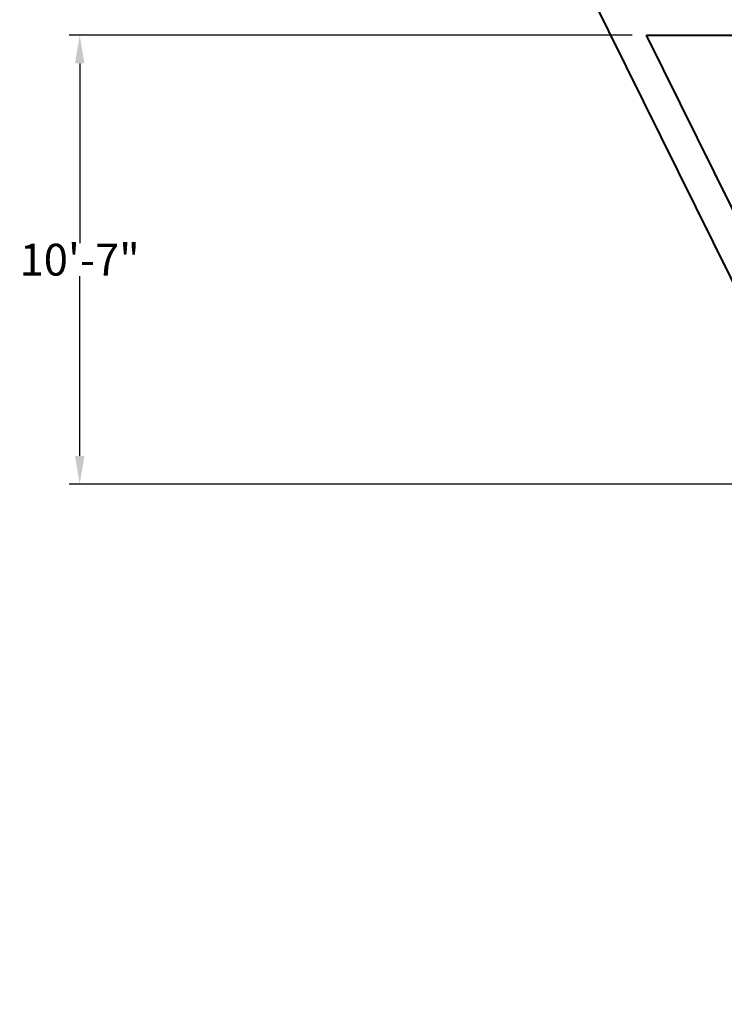
# Model space of a CAD drawing. Units: inches. Extents: x 927 to 1540, y 259 to 890.
# Tile 1 of 4: x 937 to 1137, y 303 to 582. Entities that reach past the tile are written whole.
import ezdxf

# ---------------------------------------------------------------- set-up
doc = ezdxf.new("R2010")
doc.units = ezdxf.units.IN
doc.header["$MEASUREMENT"] = 0
doc.layers.add('A-ANNO-DIMS', color=2, linetype='Continuous', lineweight=18)
doc.layers.add('A-WALL', color=7, linetype='Continuous', lineweight=40)
doc.styles.get("Standard").update_dxf_attribs({"font": 'arial.ttf'})
doc.dimstyles.get("Standard").update_dxf_attribs({"dimtxt": 9, "dimasz": 8, "dimexe": 3, "dimexo": 4, "dimgap": 0.09, "dimtad": 0, "dimtih": 1, "dimtoh": 1, "dimdec": 0, "dimzin": 0, "dimdsep": 46, "dimlunit": 3, "dimtxsty": 'Standard', "dimcen": 0.09, "dimadec": 0, "dimazin": 0, "dimtfac": 1, "dimtdec": 0, "dimtofl": 0, "dimtmove": 0, "dimatfit": 3, "dimfxl": 1, "dimtolj": 1, "dimtzin": 0, "dimarcsym": 0})

# ---------------------------------------------------------------- blocks, each defined once
blk = doc.blocks.new('*D57')
at = {"layer": 'A-ANNO-DIMS', "color": 0, "lineweight": -2, "transparency": 16777216}
for p, q in [((1110.59, 577.32), (951.4, 577.32)), ((954.4, 569.32), (954.4, 518.54)), ((954.4, 458.39), (954.4, 509.17)), ((1173.3, 450.39), (951.4, 450.39))]:
    blk.add_line(p, q, dxfattribs=at)
at = {"layer": 'A-ANNO-DIMS', "color": 0, "lineweight": 100, "transparency": 16777216}
for points in [[(953.07, 569.32), (955.74, 569.32), (954.4, 577.32)], [(953.07, 458.39), (955.74, 458.39), (954.4, 450.39)]]:
    blk.add_solid(points, dxfattribs=at)
at = {"layer": 'Defpoints', "color": 0, "lineweight": 100, "transparency": 16777216}
for p in [(1114.59, 577.32), (954.4, 450.39), (1177.3, 450.39)]:
    blk.add_point(p, dxfattribs=at)
at = {"layer": 'A-ANNO-DIMS', "color": 0, "transparency": 16777216, "insert": (954.4, 513.86), "char_height": 9, "attachment_point": 5}
blk.add_mtext('\\A1;10\'-7"', dxfattribs=at)

msp = doc.modelspace()

# ---------------------------------------------------------------- linework, layer by layer
at = {"layer": 'A-WALL'}
for p, q in [((1239.89, 303.39), (985.3, 818.67)), ((1114.59, 577.32), (1255.48, 577.32)), ((1177.3, 450.39), (1114.59, 577.32))]:
    msp.add_line(p, q, dxfattribs=at)

# ---------------------------------------------------------------- dimensions: what is measured, and where the dimension line sits
at = {"layer": 'A-ANNO-DIMS'}
dim = msp.add_linear_dim(base=(954.4, 450.39), p1=(1114.59, 577.32), p2=(1177.3, 450.39), angle=90, dimstyle='Standard', override={"dimdec": 1, "dimlfac": 1, "dimrnd": 0, "dimzin": 1, "dimdsep": 46, "dimlunit": 4, "dimfrac": 2}, dxfattribs=at)
dim.commit()
dim.dimension.update_dxf_attribs({"geometry": '*D57', "text_midpoint": (954.4, 513.86)})

doc.saveas('drawing.dxf')
